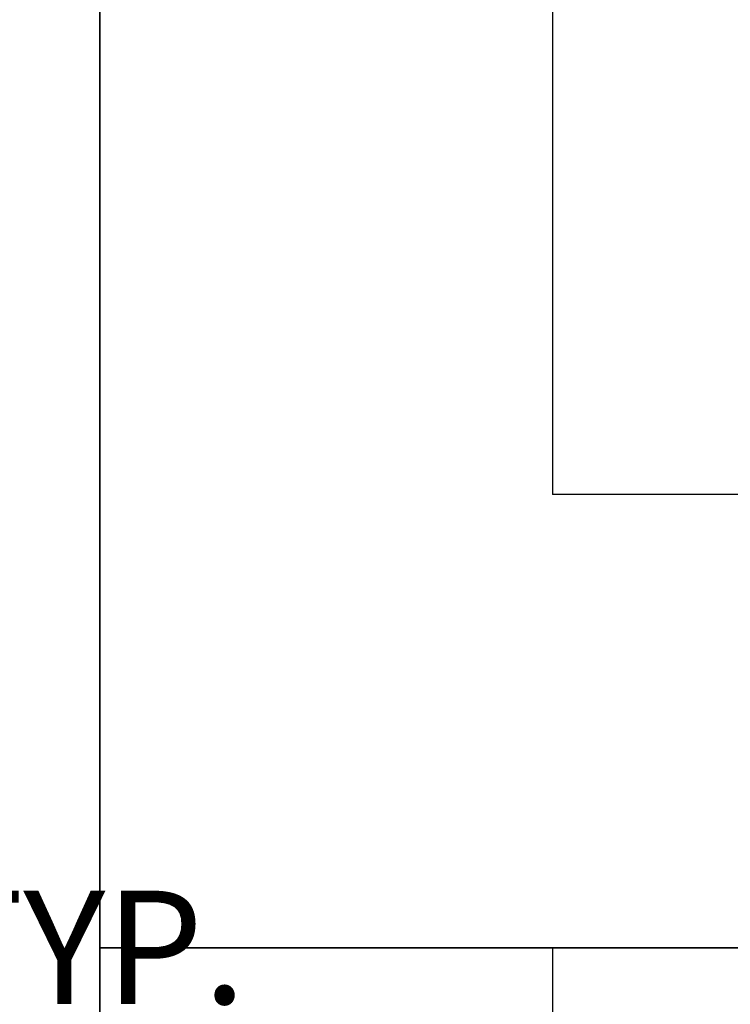
# Model space of a CAD drawing. Units: inches. Extents: x -1198 to -69, y -512 to 437.
# Tile 29 of 50: x -696 to -658, y 158 to 210. Entities that reach past the tile are written whole.
import ezdxf

# ---------------------------------------------------------------- set-up
doc = ezdxf.new("R2010")
doc.units = ezdxf.units.IN
doc.header["$MEASUREMENT"] = 0
for name, color, linetype, lineweight in [('A-ANNO-DIMS', 2, 'Continuous', 18), ('A-FLOR-CASE', 7, 'Continuous', 25), ('A-WALL', 7, 'Continuous', 35)]:
    doc.layers.add(name, color=color, linetype=linetype, lineweight=lineweight)
doc.styles.get("Standard").update_dxf_attribs({"font": 'arial.ttf'})
doc.dimstyles.get("Standard").update_dxf_attribs({"dimtxt": 6, "dimasz": 6, "dimexe": 0.18, "dimexo": 0.0625, "dimgap": 0.09, "dimtad": 0, "dimtih": 1, "dimtoh": 1, "dimdec": 0, "dimzin": 0, "dimdsep": 46, "dimlunit": 4, "dimtxsty": 'Standard', "dimblk": 'OBLIQUE', "dimcen": 0.09, "dimadec": 0, "dimazin": 0, "dimtfac": 1, "dimtdec": 0, "dimtofl": 0, "dimtmove": 0, "dimatfit": 3, "dimfxl": 1, "dimtolj": 1, "dimtzin": 0, "dimarcsym": 0})

# ---------------------------------------------------------------- blocks, each defined once
blk = doc.blocks.new('COUNTER-L')
at = {"ltscale": 10}
for p in [(0, 96), (49.349, 24)]:
    blk.add_line(p, (0, 24), dxfattribs=at)
blk = doc.blocks.new('_Oblique')
at = {"color": 0, "linetype": 'ByBlock', "lineweight": -2}
blk.add_line((-0.5, -0.5), (0.5, 0.5), dxfattribs=at)
blk = doc.blocks.new('*D34')
at = {"layer": 'A-ANNO-DIMS', "color": 0, "lineweight": -2, "ltscale": 10, "transparency": 16777216}
for p, q in [((-757.751, 165.217), (-757.751, 161.069)), ((-730.881, 165.217), (-730.881, 161.069)), ((-757.751, 161.249), (-730.881, 161.249)), ((-730.881, 161.249), (-724.881, 161.249))]:
    blk.add_line(p, q, dxfattribs=at)
at = {"layer": 'DEFPOINTS', "color": 0, "ltscale": 10, "transparency": 16777216}
for p in [(-757.751, 165.279), (-730.881, 165.279), (-730.881, 161.249)]:
    blk.add_point(p, dxfattribs=at)
at = {"layer": 'A-ANNO-DIMS', "color": 0, "lineweight": -2, "ltscale": 10, "transparency": 16777216, "xscale": 6, "yscale": 6, "zscale": 6, "rotation": 180}
blk.add_blockref('_Oblique', (-757.751, 161.249), dxfattribs=at)
at = {"layer": 'A-ANNO-DIMS', "color": 0, "lineweight": -2, "ltscale": 10, "transparency": 16777216, "xscale": 6, "yscale": 6, "zscale": 6}
blk.add_blockref('_Oblique', (-730.881, 161.249), dxfattribs=at)
at = {"layer": 'A-ANNO-DIMS', "color": 0, "ltscale": 10, "transparency": 16777216, "insert": (-703.816, 161.249), "char_height": 6, "attachment_point": 5}
blk.add_mtext('\\A1;D1 27 TYP.', dxfattribs=at)
blk = doc.blocks.new('*D57')
at = {"layer": 'A-ANNO-DIMS', "color": 0, "lineweight": -2, "ltscale": 10, "transparency": 16777216}
for p, q in [((-667.751, 161.165), (-667.751, 146.648)), ((-618.402, 161.165), (-618.402, 146.648)), ((-667.751, 146.828), (-657.89, 146.828)), ((-618.402, 146.828), (-628.263, 146.828))]:
    blk.add_line(p, q, dxfattribs=at)
at = {"layer": 'DEFPOINTS', "color": 0, "ltscale": 10, "transparency": 16777216}
for p in [(-667.751, 161.228), (-618.402, 161.228), (-618.402, 146.828)]:
    blk.add_point(p, dxfattribs=at)
at = {"layer": 'A-ANNO-DIMS', "color": 0, "lineweight": -2, "ltscale": 10, "transparency": 16777216, "xscale": 6, "yscale": 6, "zscale": 6, "rotation": 180}
blk.add_blockref('_Oblique', (-667.751, 146.828), dxfattribs=at)
at = {"layer": 'A-ANNO-DIMS', "color": 0, "lineweight": -2, "ltscale": 10, "transparency": 16777216, "xscale": 6, "yscale": 6, "zscale": 6}
blk.add_blockref('_Oblique', (-618.402, 146.828), dxfattribs=at)
at = {"layer": 'A-ANNO-DIMS', "color": 0, "ltscale": 10, "transparency": 16777216, "insert": (-643.076, 146.828), "char_height": 6, "attachment_point": 5}
blk.add_mtext('\\A1;49 TYP.', dxfattribs=at)
blk = doc.blocks.new('*D76')
at = {"layer": 'A-ANNO-DIMS', "color": 0, "lineweight": -2, "ltscale": 10, "transparency": 16777216}
for p, q in [((-711.132, -38.21), (-711.132, 433.184)), ((-711.132, 433.004), (-697.751, 433.004)), ((-697.751, -38.21), (-697.751, 433.184)), ((-697.751, 433.004), (-691.751, 433.004))]:
    blk.add_line(p, q, dxfattribs=at)
at = {"layer": 'DEFPOINTS', "color": 0, "ltscale": 10, "transparency": 16777216}
for p in [(-697.751, 433.004), (-711.132, -38.272), (-697.751, -38.272)]:
    blk.add_point(p, dxfattribs=at)
at = {"layer": 'A-ANNO-DIMS', "color": 0, "lineweight": -2, "ltscale": 10, "transparency": 16777216, "xscale": 6, "yscale": 6, "zscale": 6, "rotation": 180}
blk.add_blockref('_Oblique', (-711.132, 433.004), dxfattribs=at)
at = {"layer": 'A-ANNO-DIMS', "color": 0, "lineweight": -2, "ltscale": 10, "transparency": 16777216, "xscale": 6, "yscale": 6, "zscale": 6}
blk.add_blockref('_Oblique', (-697.751, 433.004), dxfattribs=at)
at = {"layer": 'A-ANNO-DIMS', "color": 0, "ltscale": 10, "transparency": 16777216, "insert": (-681.814, 433.004), "char_height": 6, "attachment_point": 5}
blk.add_mtext('\\A1;13.38', dxfattribs=at)

msp = doc.modelspace()

# ---------------------------------------------------------------- linework, layer by layer
at = {"layer": 'A-WALL', "ltscale": 10}
for p, q in [((-691.7509, 257.2277), (-691.7509, 38.2277)), ((-691.7509, 257.2277), (-691.7509, 161.2277)), ((-565.7509, 161.2277), (-691.7509, 161.2277))]:
    msp.add_line(p, q, dxfattribs=at)

# ---------------------------------------------------------------- block references
at = {"layer": 'A-FLOR-CASE'}
msp.add_blockref('COUNTER-L', (-667.751, 161.228), dxfattribs=at)

# ---------------------------------------------------------------- dimensions: what is measured, and where the dimension line sits
at = {"layer": 'A-ANNO-DIMS', "ltscale": 10}
dim = msp.add_linear_dim(base=(-697.7509, 433.0036), p1=(-711.1319, -38.2723), p2=(-697.7509, -38.2723), dimstyle='Standard', override={"dimdec": 2, "dimlfac": 1, "dimrnd": 0, "dimzin": 0, "dimdsep": 46, "dimlunit": 2}, dxfattribs=at)
dim.commit()
dim.dimension.update_dxf_attribs({"geometry": '*D76', "text_midpoint": (-681.8137, 433.0036)})
for base, p1, p2, text, picture, middle in [((-730.8812, 161.2489), (-757.7509, 165.2794), (-730.8812, 165.2794), 'D1 <> TYP.', '*D34', (-703.8157, 161.2489)), ((-618.4019, 146.8277), (-667.7509, 161.2277), (-618.4019, 161.2277), '<> TYP.', '*D57', (-643.0764, 146.8277))]:
    dim = msp.add_linear_dim(base=base, p1=p1, p2=p2, text=text, dimstyle='Standard', override={"dimdec": 0, "dimlfac": 1, "dimrnd": 0, "dimzin": 0, "dimdsep": 46, "dimlunit": 2}, dxfattribs=at)
    dim.commit()
    dim.dimension.update_dxf_attribs({"geometry": picture, "text_midpoint": middle})

doc.saveas('drawing.dxf')
